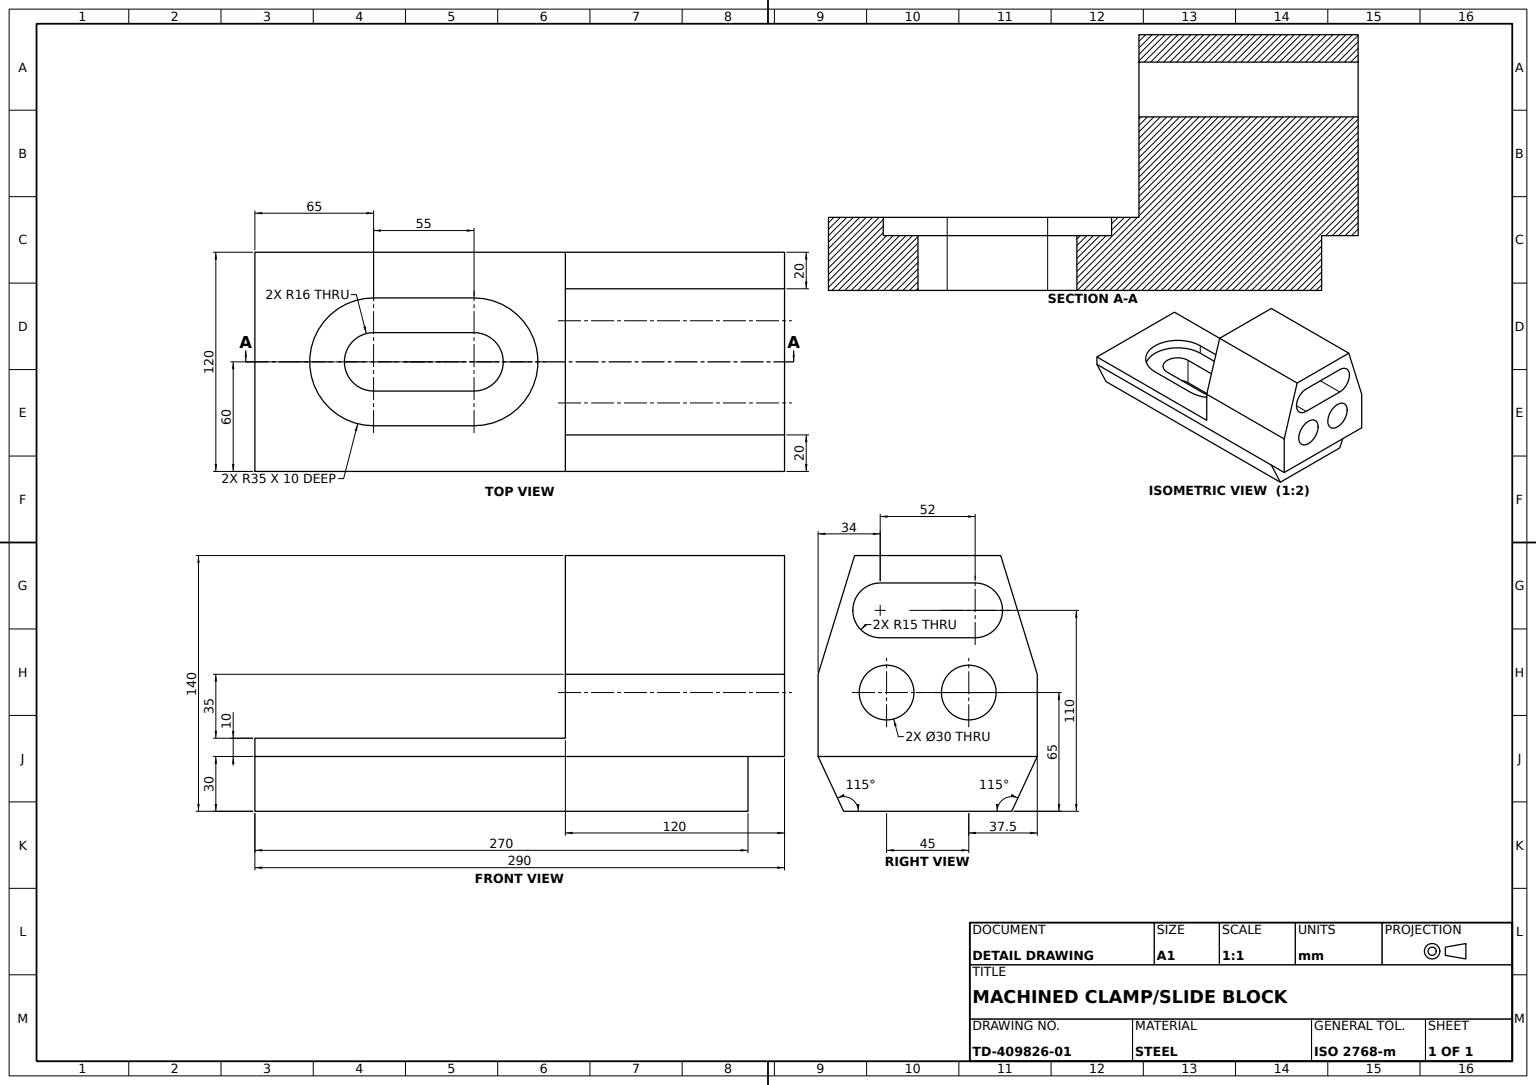
from build123d import *

# Parameters (mm, degrees)
BASE_PLATE_DEPTH              = 10
LOWER_RAIL_DEPTH              = 270
UPPER_BLOCK_DEPTH             = 120
BLOCK_HOLES_AND_SLOT_SKETCH_R = 15
BLOCK_HOLES_AND_SLOT_DEPTH    = 212
BASE_SLOT_COUNTERBORE_DEPTH   = 10
BASE_THROUGH_SLOT_DEPTH       = 68


with BuildPart() as part:
    # Base Plate Sketch → Base Plate (new body)
    with BuildSketch(Plane(origin=(0, 0, 0), x_dir=(1, 0, 0), z_dir=(0, 1, 0))):
        Polygon((145, 0), (145, 60), (-145, 60), (-145, -60), (145, -60), align=None)
    extrude(amount=BASE_PLATE_DEPTH)

    # Lower Rail Sketch → Lower Rail (add)
    with BuildSketch(Plane.ZY.offset(145)):
        Polygon((60, 0), (46.010770255, -30), (-46.010770255, -30), (-60, 0), align=None)
    extrude(amount=-LOWER_RAIL_DEPTH)

    # Upper Block Sketch → Upper Block (add)
    with BuildSketch(Plane(origin=(25, 0, 0), x_dir=(0, 0, -1), z_dir=(1, 0, 0))):
        Polygon((0, 110), (40, 110), (60, 45), (60, 10), (-60, 10), (-60, 45), (-40, 110), align=None)
    extrude(amount=UPPER_BLOCK_DEPTH)

    # Block Holes and Slot Sketch → Block Holes and Slot (cut)
    with BuildSketch(Plane.ZY.offset(-25)):
        with Locations((22.5, 35)):
            Circle(BLOCK_HOLES_AND_SLOT_SKETCH_R)
        with Locations((-22.5, 35)):
            Circle(BLOCK_HOLES_AND_SLOT_SKETCH_R)
        with BuildLine():
            Line((-26, 95), (26, 95))
            ThreePointArc((26, 95), (41, 80), (26, 65))
            Line((26, 65), (-26, 65))
            ThreePointArc((-26, 65), (-41, 80), (-26, 95))
        make_face()
    extrude(amount=-BLOCK_HOLES_AND_SLOT_DEPTH, mode=Mode.SUBTRACT)

    # Base Slot Counterbore Sketch → Base Slot Counterbore (cut)
    with BuildSketch(Plane(origin=(0, 10, 0), x_dir=(1, 0, 0), z_dir=(0, 1, 0))):
        with BuildLine():
            Line((-80, 35), (-25, 35))
            ThreePointArc((-25, 35), (10, 0), (-25, -35))
            Line((-25, -35), (-80, -35))
            ThreePointArc((-80, -35), (-115, 0), (-80, 35))
        make_face()
    extrude(amount=-BASE_SLOT_COUNTERBORE_DEPTH, mode=Mode.SUBTRACT)

    # Base Through Slot Sketch → Base Through Slot (cut)
    with BuildSketch(Plane(origin=(0, 0, 0), x_dir=(1, 0, 0), z_dir=(0, 1, 0))):
        with BuildLine():
            Line((-80, 16), (-25, 16))
            ThreePointArc((-25, 16), (-9, 0), (-25, -16))
            Line((-25, -16), (-80, -16))
            ThreePointArc((-80, -16), (-96, 0), (-80, 16))
        make_face()
    extrude(amount=-BASE_THROUGH_SLOT_DEPTH, mode=Mode.SUBTRACT)


solid = part.part
